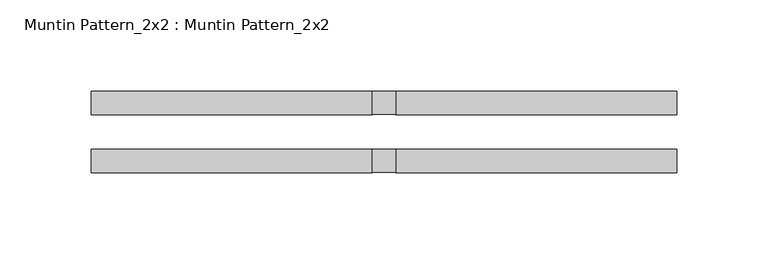
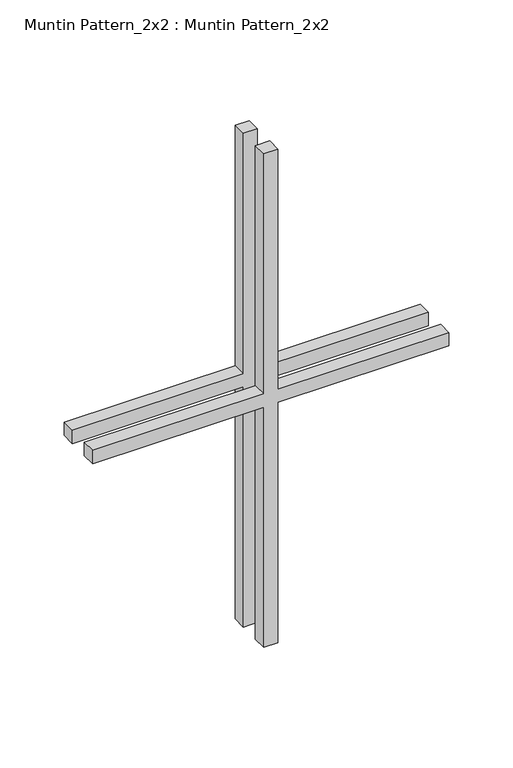
"""IFC4 building model written with IfcOpenShell, lengths in millimetres: proxy geometry, Muntin Pattern_2x2 : Muntin Pattern_2x2."""

from ifc_helpers import new_model, si_unit, frame, origin, place, context, project, spatial, polyline, outline, extrude, source, transform, mapped, element, save


def muntin_pattern_2x2_muntin_pattern_2x2_bc89accc(model_context):
    return source(origin(), model_context, "Body", "SweptSolid", [
        extrude(outline(polyline([(241.3, -6.35), (241.3, -160.3375), (228.6, -160.3375), (228.6, -6.35), (0.0, -6.35), (0.0, 6.35), (228.6, 6.35), (228.6, 160.3375), (241.3, 160.3375), (241.3, 6.35), (469.9, 6.35), (469.9, -6.35), (241.3, -6.35)])), frame((0.0, -22.225, 0.0), z_axis=(0.0, 1.0, 0.0), x_axis=(0.0, 0.0, 1.0)), (0.0, 0.0, 1.0), 12.7),
        extrude(outline(polyline([(241.3, -6.35), (241.3, -160.3375), (228.6, -160.3375), (228.6, -6.35), (0.0, -6.35), (0.0, 6.35), (228.6, 6.35), (228.6, 160.3375), (241.3, 160.3375), (241.3, 6.35), (469.9, 6.35), (469.9, -6.35), (241.3, -6.35)])), frame((0.0, 9.525, 0.0), z_axis=(0.0, 1.0, 0.0), x_axis=(0.0, 0.0, 1.0)), (0.0, 0.0, 1.0), 12.7),
    ])


if __name__ == "__main__":
    model = new_model("IFC4")
    model_context = context("Model", 3, world=origin())
    ifc_project = project(units=[si_unit("LENGTHUNIT", "METRE", prefix="MILLI")], contexts=[model_context])
    site = spatial("IfcSite", under=ifc_project)
    building = spatial("IfcBuilding", under=site)
    placement = place(None, origin())
    muntin_pattern_2x2_muntin_pattern_2x2_shape = muntin_pattern_2x2_muntin_pattern_2x2_bc89accc(model_context)
    element("IfcBuildingElementProxy", 1, Name="Muntin Pattern_2x2 : Muntin Pattern_2x2", ObjectType="Muntin Pattern_2x2 : Muntin Pattern_2x2", at=placement, inside=building, context=model_context, shape_type="MappedRepresentation", body=[
        mapped(muntin_pattern_2x2_muntin_pattern_2x2_shape, transform((0.0, 0.0, 0.0), x_axis=(1.0, 0.0, 0.0), y_axis=(0.0, 1.0, 0.0), z_axis=(0.0, 0.0, 1.0))),
    ])
    save(model, "model.ifc")

# Revit data of these elements
# Type "Muntin Pattern_2x2 : Muntin Pattern_2x2"
#   Width [instance default] = 48"
#   Thickness = 0.5"
#   Height [instance default] = 48"
#   Distance = 0.75"
#   Interior Material [instance default] = none
#   Exterior Material [instance default] = none
#   Default Elevation = 0
# Element 1 (IfcBuildingElementProxy, "Muntin Pattern_2x2 : Muntin Pattern_2x2")
#   Width = 12.625"
#   Height = 18.5"
#   Interior Material = Wood - Stained
#   Exterior Material = Clad - White
#   Materials on its faces: "Clad - White", "Wood - Stained"
# Materials
#   "Clad - White": class "Wood", colour RGB 242 242 238, transparency 0, Cost = 0
#   "Wood - Stained": class "Wood", colour RGB 224 178 126, transparency 0, Cost = 0
